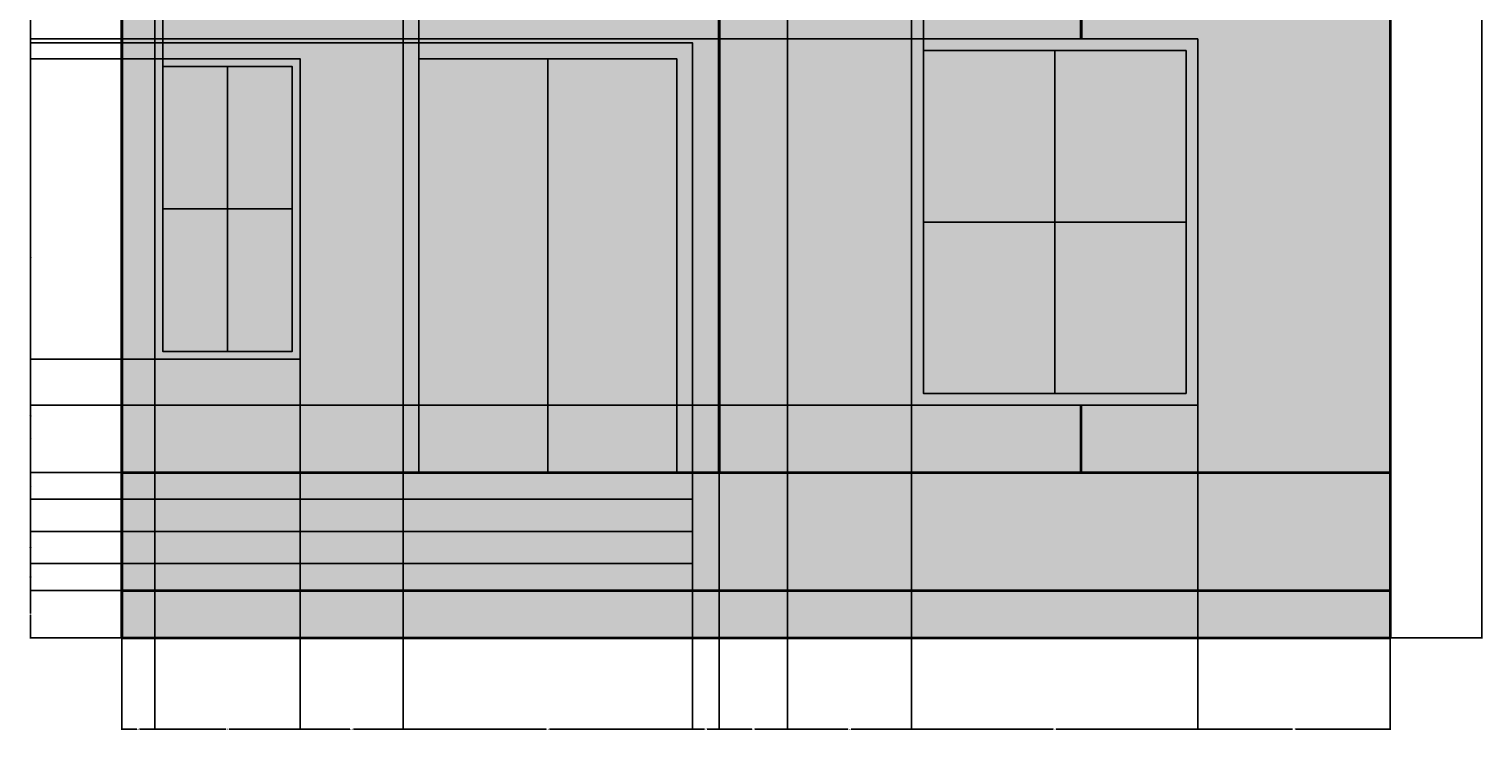
# Model space of a CAD drawing. Units: feet. Extents: x 2368 to 2738, y 1285 to 1782.
# Tile 1 of 6: x 2368 to 2738, y 1285 to 1464. Entities that reach past the tile are written whole.
import ezdxf

# ---------------------------------------------------------------- set-up
doc = ezdxf.new("R2010")
doc.units = ezdxf.units.FT
for name, color, linetype, lineweight in [('A-ANNO-DIMS', 2, 'Continuous', 18), ('A-DOOR', 3, 'Continuous', 25), ('A-ELEV', 7, 'Continuous', 35), ('A-ELEV-PATT', 252, 'Continuous', 13), ('A-FLOR-STRS', 2, 'Continuous', 25), ('A-GLAZ', 4, 'Continuous', 25)]:
    doc.layers.add(name, color=color, linetype=linetype, lineweight=lineweight)
doc.styles.get("Standard").update_dxf_attribs({"font": 'arial.ttf'})
doc.dimstyles.get("Standard").update_dxf_attribs({"dimtxt": 0.18, "dimasz": 0.18, "dimexe": 0.18, "dimexo": 0.0625, "dimgap": 0.09, "dimtad": 0, "dimtih": 1, "dimtoh": 1, "dimdec": 1, "dimzin": 0, "dimdsep": 46, "dimlunit": 3, "dimtxsty": 'Standard', "dimcen": 0.09, "dimadec": 0, "dimazin": 0, "dimtfac": 1, "dimtdec": 1, "dimtofl": 0, "dimtmove": 0, "dimatfit": 3, "dimfxl": 1, "dimtolj": 1, "dimtzin": 0, "dimarcsym": 0})

# ---------------------------------------------------------------- blocks, each defined once
blk = doc.blocks.new('*D2')
at = {"layer": 'A-ANNO-DIMS', "color": 0, "lineweight": -2, "transparency": 16777216}
for p, q in [((2714.23, 1758.68), (2737.59, 1758.68)), ((2737.41, 1758.5), (2737.41, 1533.95)), ((2737.41, 1309.04), (2737.41, 1533.58)), ((2714.23, 1308.86), (2737.59, 1308.86))]:
    blk.add_line(p, q, dxfattribs=at)
at = {"layer": 'A-ANNO-DIMS', "color": 0, "transparency": 16777216}
for points in [[(2737.38, 1758.5), (2737.44, 1758.5), (2737.41, 1758.68)], [(2737.38, 1309.04), (2737.44, 1309.04), (2737.41, 1308.86)]]:
    blk.add_solid(points, dxfattribs=at)
at = {"layer": 'Defpoints', "color": 0, "transparency": 16777216}
for p in [(2714.16, 1758.68), (2737.41, 1758.68), (2714.16, 1308.86)]:
    blk.add_point(p, dxfattribs=at)
at = {"layer": 'A-ANNO-DIMS', "color": 0, "transparency": 16777216, "insert": (2737.41, 1533.77), "char_height": 0.18, "attachment_point": 5}
blk.add_mtext('\\A1;449.8', dxfattribs=at)
blk = doc.blocks.new('*D3')
at = {"layer": 'A-ANNO-DIMS', "color": 0, "lineweight": -2, "transparency": 16777216}
for p, q in [((2391.48, 1320.86), (2368.11, 1320.86)), ((2368.29, 1320.68), (2368.29, 1315.04)), ((2368.29, 1309.04), (2368.29, 1314.67)), ((2391.48, 1308.86), (2368.11, 1308.86))]:
    blk.add_line(p, q, dxfattribs=at)
at = {"layer": 'A-ANNO-DIMS', "color": 0, "transparency": 16777216}
for points in [[(2368.26, 1320.68), (2368.32, 1320.68), (2368.29, 1320.86)], [(2368.26, 1309.04), (2368.32, 1309.04), (2368.29, 1308.86)]]:
    blk.add_solid(points, dxfattribs=at)
at = {"layer": 'Defpoints', "color": 0, "transparency": 16777216}
for p in [(2368.29, 1320.86), (2391.54, 1320.86), (2391.54, 1308.86)]:
    blk.add_point(p, dxfattribs=at)
at = {"layer": 'A-ANNO-DIMS', "color": 0, "transparency": 16777216, "insert": (2368.29, 1314.86), "char_height": 0.18, "attachment_point": 5}
blk.add_mtext('\\A1;12', dxfattribs=at)
blk = doc.blocks.new('*D4')
at = {"layer": 'A-ANNO-DIMS', "color": 0, "lineweight": -2, "transparency": 16777216}
for p, q in [((2391.48, 1350.86), (2368.11, 1350.86)), ((2368.29, 1350.68), (2368.29, 1336.04)), ((2368.29, 1321.04), (2368.29, 1335.67)), ((2391.48, 1320.86), (2368.11, 1320.86))]:
    blk.add_line(p, q, dxfattribs=at)
at = {"layer": 'A-ANNO-DIMS', "color": 0, "transparency": 16777216}
for points in [[(2368.26, 1350.68), (2368.32, 1350.68), (2368.29, 1350.86)], [(2368.26, 1321.04), (2368.32, 1321.04), (2368.29, 1320.86)]]:
    blk.add_solid(points, dxfattribs=at)
at = {"layer": 'Defpoints', "color": 0, "transparency": 16777216}
for p in [(2368.29, 1350.86), (2391.54, 1350.86), (2391.54, 1320.86)]:
    blk.add_point(p, dxfattribs=at)
at = {"layer": 'A-ANNO-DIMS', "color": 0, "transparency": 16777216, "insert": (2368.29, 1335.86), "char_height": 0.18, "attachment_point": 5}
blk.add_mtext('\\A1;30', dxfattribs=at)
blk = doc.blocks.new('*D5')
at = {"layer": 'A-ANNO-DIMS', "color": 0, "lineweight": -2, "transparency": 16777216}
for p, q in [((2399.84, 1379.67), (2368.11, 1379.67)), ((2368.29, 1379.49), (2368.29, 1365.44)), ((2368.29, 1351.04), (2368.29, 1365.08)), ((2391.48, 1350.86), (2368.11, 1350.86))]:
    blk.add_line(p, q, dxfattribs=at)
at = {"layer": 'A-ANNO-DIMS', "color": 0, "transparency": 16777216}
for points in [[(2368.26, 1379.49), (2368.32, 1379.49), (2368.29, 1379.67)], [(2368.26, 1351.04), (2368.32, 1351.04), (2368.29, 1350.86)]]:
    blk.add_solid(points, dxfattribs=at)
at = {"layer": 'Defpoints', "color": 0, "transparency": 16777216}
for p in [(2368.29, 1379.67), (2399.91, 1379.67), (2391.54, 1350.86)]:
    blk.add_point(p, dxfattribs=at)
at = {"layer": 'A-ANNO-DIMS', "color": 0, "transparency": 16777216, "insert": (2368.29, 1365.26), "char_height": 0.18, "attachment_point": 5}
blk.add_mtext('\\A1;28.814', dxfattribs=at)
blk = doc.blocks.new('*D6')
at = {"layer": 'A-ANNO-DIMS', "color": 0, "lineweight": -2, "transparency": 16777216}
for p, q in [((2391.48, 1482.86), (2368.11, 1482.86)), ((2368.29, 1482.68), (2368.29, 1469.65)), ((2368.29, 1456.26), (2368.29, 1469.29)), ((2399.84, 1456.08), (2368.11, 1456.08))]:
    blk.add_line(p, q, dxfattribs=at)
at = {"layer": 'A-ANNO-DIMS', "color": 0, "transparency": 16777216}
for points in [[(2368.26, 1482.68), (2368.32, 1482.68), (2368.29, 1482.86)], [(2368.26, 1456.26), (2368.32, 1456.26), (2368.29, 1456.08)]]:
    blk.add_solid(points, dxfattribs=at)
at = {"layer": 'Defpoints', "color": 0, "transparency": 16777216}
for p in [(2368.29, 1482.86), (2391.54, 1482.86), (2399.91, 1456.08)]:
    blk.add_point(p, dxfattribs=at)
at = {"layer": 'A-ANNO-DIMS', "color": 0, "transparency": 16777216, "insert": (2368.29, 1469.47), "char_height": 0.18, "attachment_point": 5}
blk.add_mtext('\\A1;26.77', dxfattribs=at)
blk = doc.blocks.new('*D14')
at = {"layer": 'A-ANNO-DIMS', "color": 0, "lineweight": -2, "transparency": 16777216}
for p, q in [((2399.91, 1379.61), (2399.91, 1285.43)), ((2391.54, 1350.79), (2391.54, 1285.43)), ((2391.72, 1285.61), (2395.33, 1285.61)), ((2399.73, 1285.61), (2396.12, 1285.61))]:
    blk.add_line(p, q, dxfattribs=at)
at = {"layer": 'A-ANNO-DIMS', "color": 0, "transparency": 16777216}
for points in [[(2391.72, 1285.64), (2391.72, 1285.58), (2391.54, 1285.61)], [(2399.73, 1285.64), (2399.73, 1285.58), (2399.91, 1285.61)]]:
    blk.add_solid(points, dxfattribs=at)
at = {"layer": 'Defpoints', "color": 0, "transparency": 16777216}
for p in [(2399.91, 1379.67), (2391.54, 1350.86), (2399.91, 1285.61)]:
    blk.add_point(p, dxfattribs=at)
at = {"layer": 'A-ANNO-DIMS', "color": 0, "transparency": 16777216, "insert": (2395.72, 1285.61), "char_height": 0.18, "attachment_point": 5}
blk.add_mtext('\\A1;8.365', dxfattribs=at)
blk = doc.blocks.new('*D15')
at = {"layer": 'A-ANNO-DIMS', "color": 0, "lineweight": -2, "transparency": 16777216}
for p, q in [((2399.91, 1379.61), (2399.91, 1285.43)), ((2436.85, 1379.61), (2436.85, 1285.43)), ((2400.09, 1285.61), (2417.98, 1285.61)), ((2436.67, 1285.61), (2418.77, 1285.61))]:
    blk.add_line(p, q, dxfattribs=at)
at = {"layer": 'A-ANNO-DIMS', "color": 0, "transparency": 16777216}
for points in [[(2400.09, 1285.64), (2400.09, 1285.58), (2399.91, 1285.61)], [(2436.67, 1285.64), (2436.67, 1285.58), (2436.85, 1285.61)]]:
    blk.add_solid(points, dxfattribs=at)
at = {"layer": 'Defpoints', "color": 0, "transparency": 16777216}
for p in [(2399.91, 1379.67), (2436.85, 1379.67), (2436.85, 1285.61)]:
    blk.add_point(p, dxfattribs=at)
at = {"layer": 'A-ANNO-DIMS', "color": 0, "transparency": 16777216, "insert": (2418.38, 1285.61), "char_height": 0.18, "attachment_point": 5}
blk.add_mtext('\\A1;36.94', dxfattribs=at)
blk = doc.blocks.new('*D16')
at = {"layer": 'A-ANNO-DIMS', "color": 0, "lineweight": -2, "transparency": 16777216}
for p, q in [((2436.85, 1379.61), (2436.85, 1285.43)), ((2463.03, 1350.79), (2463.03, 1285.43)), ((2437.03, 1285.61), (2449.48, 1285.61)), ((2462.85, 1285.61), (2450.41, 1285.61))]:
    blk.add_line(p, q, dxfattribs=at)
at = {"layer": 'A-ANNO-DIMS', "color": 0, "transparency": 16777216}
for points in [[(2437.03, 1285.64), (2437.03, 1285.58), (2436.85, 1285.61)], [(2462.85, 1285.64), (2462.85, 1285.58), (2463.03, 1285.61)]]:
    blk.add_solid(points, dxfattribs=at)
at = {"layer": 'Defpoints', "color": 0, "transparency": 16777216}
for p in [(2436.85, 1379.67), (2463.03, 1350.86), (2463.03, 1285.61)]:
    blk.add_point(p, dxfattribs=at)
at = {"layer": 'A-ANNO-DIMS', "color": 0, "transparency": 16777216, "insert": (2449.94, 1285.61), "char_height": 0.18, "attachment_point": 5}
blk.add_mtext('\\A1;26.184', dxfattribs=at)
blk = doc.blocks.new('*D17')
at = {"layer": 'A-ANNO-DIMS', "color": 0, "lineweight": -2, "transparency": 16777216}
for p, q in [((2463.03, 1350.79), (2463.03, 1285.43)), ((2536.68, 1350.79), (2536.68, 1285.43)), ((2463.21, 1285.61), (2499.46, 1285.61)), ((2536.5, 1285.61), (2500.25, 1285.61))]:
    blk.add_line(p, q, dxfattribs=at)
at = {"layer": 'A-ANNO-DIMS', "color": 0, "transparency": 16777216}
for points in [[(2463.21, 1285.64), (2463.21, 1285.58), (2463.03, 1285.61)], [(2536.5, 1285.64), (2536.5, 1285.58), (2536.68, 1285.61)]]:
    blk.add_solid(points, dxfattribs=at)
at = {"layer": 'Defpoints', "color": 0, "transparency": 16777216}
for p in [(2463.03, 1350.86), (2536.68, 1350.86), (2536.68, 1285.61)]:
    blk.add_point(p, dxfattribs=at)
at = {"layer": 'A-ANNO-DIMS', "color": 0, "transparency": 16777216, "insert": (2499.85, 1285.61), "char_height": 0.18, "attachment_point": 5}
blk.add_mtext('\\A1;73.64', dxfattribs=at)
blk = doc.blocks.new('*D18')
at = {"layer": 'A-ANNO-DIMS', "color": 0, "lineweight": -2, "transparency": 16777216}
for p, q in [((2536.68, 1350.79), (2536.68, 1285.43)), ((2543.45, 1350.79), (2543.45, 1285.43)), ((2536.86, 1285.61), (2539.74, 1285.61)), ((2543.27, 1285.61), (2540.39, 1285.61))]:
    blk.add_line(p, q, dxfattribs=at)
at = {"layer": 'A-ANNO-DIMS', "color": 0, "transparency": 16777216}
for points in [[(2536.86, 1285.64), (2536.86, 1285.58), (2536.68, 1285.61)], [(2543.27, 1285.64), (2543.27, 1285.58), (2543.45, 1285.61)]]:
    blk.add_solid(points, dxfattribs=at)
at = {"layer": 'Defpoints', "color": 0, "transparency": 16777216}
for p in [(2536.68, 1350.86), (2543.45, 1350.86), (2543.45, 1285.61)]:
    blk.add_point(p, dxfattribs=at)
at = {"layer": 'A-ANNO-DIMS', "color": 0, "transparency": 16777216, "insert": (2540.06, 1285.61), "char_height": 0.18, "attachment_point": 5}
blk.add_mtext('\\A1;6.77', dxfattribs=at)
blk = doc.blocks.new('*D19')
at = {"layer": 'A-ANNO-DIMS', "color": 0, "lineweight": -2, "transparency": 16777216}
for p, q in [((2560.8, 1466.04), (2560.8, 1285.43)), ((2543.45, 1350.79), (2543.45, 1285.43)), ((2543.63, 1285.61), (2551.74, 1285.61)), ((2560.62, 1285.61), (2552.51, 1285.61))]:
    blk.add_line(p, q, dxfattribs=at)
at = {"layer": 'A-ANNO-DIMS', "color": 0, "transparency": 16777216}
for points in [[(2543.63, 1285.64), (2543.63, 1285.58), (2543.45, 1285.61)], [(2560.62, 1285.64), (2560.62, 1285.58), (2560.8, 1285.61)]]:
    blk.add_solid(points, dxfattribs=at)
at = {"layer": 'Defpoints', "color": 0, "transparency": 16777216}
for p in [(2560.8, 1466.1), (2543.45, 1350.86), (2560.8, 1285.61)]:
    blk.add_point(p, dxfattribs=at)
at = {"layer": 'A-ANNO-DIMS', "color": 0, "transparency": 16777216, "insert": (2552.12, 1285.61), "char_height": 0.18, "attachment_point": 5}
blk.add_mtext('\\A1;17.35', dxfattribs=at)
blk = doc.blocks.new('*D20')
at = {"layer": 'A-ANNO-DIMS', "color": 0, "lineweight": -2, "transparency": 16777216}
for p, q in [((2560.8, 1466.04), (2560.8, 1285.43)), ((2592.41, 1367.92), (2592.41, 1285.43)), ((2560.98, 1285.61), (2576.21, 1285.61)), ((2592.23, 1285.61), (2577, 1285.61))]:
    blk.add_line(p, q, dxfattribs=at)
at = {"layer": 'A-ANNO-DIMS', "color": 0, "transparency": 16777216}
for points in [[(2560.98, 1285.64), (2560.98, 1285.58), (2560.8, 1285.61)], [(2592.23, 1285.64), (2592.23, 1285.58), (2592.41, 1285.61)]]:
    blk.add_solid(points, dxfattribs=at)
at = {"layer": 'Defpoints', "color": 0, "transparency": 16777216}
for p in [(2560.8, 1466.1), (2592.41, 1367.98), (2592.41, 1285.61)]:
    blk.add_point(p, dxfattribs=at)
at = {"layer": 'A-ANNO-DIMS', "color": 0, "transparency": 16777216, "insert": (2576.6, 1285.61), "char_height": 0.18, "attachment_point": 5}
blk.add_mtext('\\A1;31.62', dxfattribs=at)
blk = doc.blocks.new('*D21')
at = {"layer": 'A-ANNO-DIMS', "color": 0, "lineweight": -2, "transparency": 16777216}
for p, q in [((2592.41, 1367.92), (2592.41, 1285.43)), ((2665.2, 1367.92), (2665.2, 1285.43)), ((2592.59, 1285.61), (2628.41, 1285.61)), ((2665.02, 1285.61), (2629.2, 1285.61))]:
    blk.add_line(p, q, dxfattribs=at)
at = {"layer": 'A-ANNO-DIMS', "color": 0, "transparency": 16777216}
for points in [[(2592.59, 1285.64), (2592.59, 1285.58), (2592.41, 1285.61)], [(2665.02, 1285.64), (2665.02, 1285.58), (2665.2, 1285.61)]]:
    blk.add_solid(points, dxfattribs=at)
at = {"layer": 'Defpoints', "color": 0, "transparency": 16777216}
for p in [(2592.41, 1367.98), (2665.2, 1367.98), (2665.2, 1285.61)]:
    blk.add_point(p, dxfattribs=at)
at = {"layer": 'A-ANNO-DIMS', "color": 0, "transparency": 16777216, "insert": (2628.8, 1285.61), "char_height": 0.18, "attachment_point": 5}
blk.add_mtext('\\A1;72.78', dxfattribs=at)
blk = doc.blocks.new('*D22')
at = {"layer": 'A-ANNO-DIMS', "color": 0, "lineweight": -2, "transparency": 16777216}
for p, q in [((2665.2, 1367.92), (2665.2, 1285.43)), ((2714.16, 1350.79), (2714.16, 1285.43)), ((2665.38, 1285.61), (2689.28, 1285.61)), ((2713.98, 1285.61), (2690.08, 1285.61))]:
    blk.add_line(p, q, dxfattribs=at)
at = {"layer": 'A-ANNO-DIMS', "color": 0, "transparency": 16777216}
for points in [[(2665.38, 1285.64), (2665.38, 1285.58), (2665.2, 1285.61)], [(2713.98, 1285.64), (2713.98, 1285.58), (2714.16, 1285.61)]]:
    blk.add_solid(points, dxfattribs=at)
at = {"layer": 'Defpoints', "color": 0, "transparency": 16777216}
for p in [(2665.2, 1367.98), (2714.16, 1350.86), (2714.16, 1285.61)]:
    blk.add_point(p, dxfattribs=at)
at = {"layer": 'A-ANNO-DIMS', "color": 0, "transparency": 16777216, "insert": (2689.68, 1285.61), "char_height": 0.18, "attachment_point": 5}
blk.add_mtext('\\A1;48.97', dxfattribs=at)
blk = doc.blocks.new('*D23')
at = {"layer": 'A-ANNO-DIMS', "color": 0, "lineweight": -2, "transparency": 16777216}
for p, q in [((2399.84, 1456.08), (2368.11, 1456.08)), ((2368.29, 1455.9), (2368.29, 1418.06)), ((2368.29, 1379.85), (2368.29, 1417.69)), ((2399.84, 1379.67), (2368.11, 1379.67))]:
    blk.add_line(p, q, dxfattribs=at)
at = {"layer": 'A-ANNO-DIMS', "color": 0, "transparency": 16777216}
for points in [[(2368.26, 1455.9), (2368.32, 1455.9), (2368.29, 1456.08)], [(2368.26, 1379.85), (2368.32, 1379.85), (2368.29, 1379.67)]]:
    blk.add_solid(points, dxfattribs=at)
at = {"layer": 'Defpoints', "color": 0, "transparency": 16777216}
for p in [(2368.29, 1456.08), (2399.91, 1456.08), (2399.91, 1379.67)]:
    blk.add_point(p, dxfattribs=at)
at = {"layer": 'A-ANNO-DIMS', "color": 0, "transparency": 16777216, "insert": (2368.29, 1417.88), "char_height": 0.18, "attachment_point": 5}
blk.add_mtext('\\A1;76.42', dxfattribs=at)
blk = doc.blocks.new('*D24')
at = {"layer": 'A-ANNO-DIMS', "color": 0, "lineweight": -2, "transparency": 16777216}
for p, q in [((2399.91, 1456.15), (2399.91, 1782.11)), ((2400.09, 1781.93), (2400.76, 1781.93)), ((2401.73, 1781.93), (2401.06, 1781.93)), ((2401.91, 1454.15), (2401.91, 1782.11))]:
    blk.add_line(p, q, dxfattribs=at)
at = {"layer": 'A-ANNO-DIMS', "color": 0, "transparency": 16777216}
for points in [[(2400.09, 1781.96), (2400.09, 1781.9), (2399.91, 1781.93)], [(2401.73, 1781.96), (2401.73, 1781.9), (2401.91, 1781.93)]]:
    blk.add_solid(points, dxfattribs=at)
at = {"layer": 'Defpoints', "color": 0, "transparency": 16777216}
for p in [(2401.91, 1781.93), (2399.91, 1456.08), (2401.91, 1454.08)]:
    blk.add_point(p, dxfattribs=at)
at = {"layer": 'A-ANNO-DIMS', "color": 0, "transparency": 16777216, "insert": (2400.91, 1781.93), "char_height": 0.18, "attachment_point": 5}
blk.add_mtext('\\A1;2', dxfattribs=at)
blk = doc.blocks.new('*D25')
at = {"layer": 'A-ANNO-DIMS', "color": 0, "lineweight": -2, "transparency": 16777216}
for p, q in [((2462.97, 1327.76), (2368.11, 1327.76)), ((2368.29, 1327.58), (2368.29, 1324.49)), ((2368.29, 1321.04), (2368.29, 1324.12)), ((2462.97, 1320.86), (2368.11, 1320.86))]:
    blk.add_line(p, q, dxfattribs=at)
at = {"layer": 'A-ANNO-DIMS', "color": 0, "transparency": 16777216}
for points in [[(2368.26, 1327.58), (2368.32, 1327.58), (2368.29, 1327.76)], [(2368.26, 1321.04), (2368.32, 1321.04), (2368.29, 1320.86)]]:
    blk.add_solid(points, dxfattribs=at)
at = {"layer": 'Defpoints', "color": 0, "transparency": 16777216}
for p in [(2368.29, 1327.76), (2463.03, 1327.76), (2463.03, 1320.86)]:
    blk.add_point(p, dxfattribs=at)
at = {"layer": 'A-ANNO-DIMS', "color": 0, "transparency": 16777216, "insert": (2368.29, 1324.31), "char_height": 0.18, "attachment_point": 5}
blk.add_mtext('\\A1;6.901', dxfattribs=at)
blk = doc.blocks.new('*D26')
at = {"layer": 'A-ANNO-DIMS', "color": 0, "lineweight": -2, "transparency": 16777216}
for p, q in [((2462.97, 1335.86), (2368.11, 1335.86)), ((2368.29, 1335.68), (2368.29, 1331.99)), ((2368.29, 1327.94), (2368.29, 1331.62)), ((2462.97, 1327.76), (2368.11, 1327.76))]:
    blk.add_line(p, q, dxfattribs=at)
at = {"layer": 'A-ANNO-DIMS', "color": 0, "transparency": 16777216}
for points in [[(2368.26, 1335.68), (2368.32, 1335.68), (2368.29, 1335.86)], [(2368.26, 1327.94), (2368.32, 1327.94), (2368.29, 1327.76)]]:
    blk.add_solid(points, dxfattribs=at)
at = {"layer": 'Defpoints', "color": 0, "transparency": 16777216}
for p in [(2368.29, 1335.86), (2463.03, 1335.86), (2463.03, 1327.76)]:
    blk.add_point(p, dxfattribs=at)
at = {"layer": 'A-ANNO-DIMS', "color": 0, "transparency": 16777216, "insert": (2368.29, 1331.81), "char_height": 0.18, "attachment_point": 5}
blk.add_mtext('\\A1;8.099', dxfattribs=at)
blk = doc.blocks.new('*D27')
at = {"layer": 'A-ANNO-DIMS', "color": 0, "lineweight": -2, "transparency": 16777216}
for p, q in [((2462.97, 1344.11), (2368.11, 1344.11)), ((2368.29, 1343.93), (2368.29, 1340.17)), ((2368.29, 1336.04), (2368.29, 1339.8)), ((2462.97, 1335.86), (2368.11, 1335.86))]:
    blk.add_line(p, q, dxfattribs=at)
at = {"layer": 'A-ANNO-DIMS', "color": 0, "transparency": 16777216}
for points in [[(2368.26, 1343.93), (2368.32, 1343.93), (2368.29, 1344.11)], [(2368.26, 1336.04), (2368.32, 1336.04), (2368.29, 1335.86)]]:
    blk.add_solid(points, dxfattribs=at)
at = {"layer": 'Defpoints', "color": 0, "transparency": 16777216}
for p in [(2368.29, 1344.11), (2463.03, 1344.11), (2463.03, 1335.86)]:
    blk.add_point(p, dxfattribs=at)
at = {"layer": 'A-ANNO-DIMS', "color": 0, "transparency": 16777216, "insert": (2368.29, 1339.98), "char_height": 0.18, "attachment_point": 5}
blk.add_mtext('\\A1;8.258', dxfattribs=at)
blk = doc.blocks.new('*D28')
at = {"layer": 'A-ANNO-DIMS', "color": 0, "lineweight": -2, "transparency": 16777216}
for p, q in [((2462.97, 1350.86), (2368.11, 1350.86)), ((2368.29, 1350.68), (2368.29, 1347.67)), ((2368.29, 1344.29), (2368.29, 1347.3)), ((2462.97, 1344.11), (2368.11, 1344.11))]:
    blk.add_line(p, q, dxfattribs=at)
at = {"layer": 'A-ANNO-DIMS', "color": 0, "transparency": 16777216}
for points in [[(2368.26, 1350.68), (2368.32, 1350.68), (2368.29, 1350.86)], [(2368.26, 1344.29), (2368.32, 1344.29), (2368.29, 1344.11)]]:
    blk.add_solid(points, dxfattribs=at)
at = {"layer": 'Defpoints', "color": 0, "transparency": 16777216}
for p in [(2368.29, 1350.86), (2463.03, 1350.86), (2463.03, 1344.11)]:
    blk.add_point(p, dxfattribs=at)
at = {"layer": 'A-ANNO-DIMS', "color": 0, "transparency": 16777216, "insert": (2368.29, 1347.48), "char_height": 0.18, "attachment_point": 5}
blk.add_mtext('\\A1;6.742', dxfattribs=at)
blk = doc.blocks.new('*D29')
at = {"layer": 'A-ANNO-DIMS', "color": 0, "lineweight": -2, "transparency": 16777216}
for p, q in [((2462.97, 1460.1), (2368.11, 1460.1)), ((2368.29, 1459.92), (2368.29, 1405.66)), ((2368.29, 1351.04), (2368.29, 1405.29)), ((2462.97, 1350.86), (2368.11, 1350.86))]:
    blk.add_line(p, q, dxfattribs=at)
at = {"layer": 'A-ANNO-DIMS', "color": 0, "transparency": 16777216}
for points in [[(2368.26, 1459.92), (2368.32, 1459.92), (2368.29, 1460.1)], [(2368.26, 1351.04), (2368.32, 1351.04), (2368.29, 1350.86)]]:
    blk.add_solid(points, dxfattribs=at)
at = {"layer": 'Defpoints', "color": 0, "transparency": 16777216}
for p in [(2368.29, 1460.1), (2463.03, 1460.1), (2463.03, 1350.86)]:
    blk.add_point(p, dxfattribs=at)
at = {"layer": 'A-ANNO-DIMS', "color": 0, "transparency": 16777216, "insert": (2368.29, 1405.48), "char_height": 0.18, "attachment_point": 5}
blk.add_mtext('\\A1;109.24', dxfattribs=at)
blk = doc.blocks.new('*D30')
at = {"layer": 'A-ANNO-DIMS', "color": 0, "lineweight": -2, "transparency": 16777216}
for p, q in [((2463.03, 1460.16), (2463.03, 1782.11)), ((2463.21, 1781.93), (2464.88, 1781.93)), ((2466.85, 1781.93), (2465.18, 1781.93)), ((2467.03, 1456.16), (2467.03, 1782.11))]:
    blk.add_line(p, q, dxfattribs=at)
at = {"layer": 'A-ANNO-DIMS', "color": 0, "transparency": 16777216}
for points in [[(2463.21, 1781.96), (2463.21, 1781.9), (2463.03, 1781.93)], [(2466.85, 1781.96), (2466.85, 1781.9), (2467.03, 1781.93)]]:
    blk.add_solid(points, dxfattribs=at)
at = {"layer": 'Defpoints', "color": 0, "transparency": 16777216}
for p in [(2467.03, 1781.93), (2463.03, 1460.1), (2467.03, 1456.1)]:
    blk.add_point(p, dxfattribs=at)
at = {"layer": 'A-ANNO-DIMS', "color": 0, "transparency": 16777216, "insert": (2465.03, 1781.93), "char_height": 0.18, "attachment_point": 5}
blk.add_mtext('\\A1;4', dxfattribs=at)
blk = doc.blocks.new('*D31')
at = {"layer": 'A-ANNO-DIMS', "color": 0, "lineweight": -2, "transparency": 16777216}
for p, q in [((2592.35, 1367.98), (2368.11, 1367.98)), ((2368.29, 1367.8), (2368.29, 1359.6)), ((2368.29, 1351.04), (2368.29, 1359.24)), ((2635.43, 1350.86), (2368.11, 1350.86))]:
    blk.add_line(p, q, dxfattribs=at)
at = {"layer": 'A-ANNO-DIMS', "color": 0, "transparency": 16777216}
for points in [[(2368.26, 1367.8), (2368.32, 1367.8), (2368.29, 1367.98)], [(2368.26, 1351.04), (2368.32, 1351.04), (2368.29, 1350.86)]]:
    blk.add_solid(points, dxfattribs=at)
at = {"layer": 'Defpoints', "color": 0, "transparency": 16777216}
for p in [(2368.29, 1367.98), (2592.41, 1367.98), (2635.49, 1350.86)]:
    blk.add_point(p, dxfattribs=at)
at = {"layer": 'A-ANNO-DIMS', "color": 0, "transparency": 16777216, "insert": (2368.29, 1359.42), "char_height": 0.18, "attachment_point": 5}
blk.add_mtext('\\A1;17.13', dxfattribs=at)
blk = doc.blocks.new('*D32')
at = {"layer": 'A-ANNO-DIMS', "color": 0, "lineweight": -2, "transparency": 16777216}
for p, q in [((2592.35, 1461.14), (2368.11, 1461.14)), ((2368.29, 1460.96), (2368.29, 1414.74)), ((2368.29, 1368.16), (2368.29, 1414.38)), ((2592.35, 1367.98), (2368.11, 1367.98))]:
    blk.add_line(p, q, dxfattribs=at)
at = {"layer": 'A-ANNO-DIMS', "color": 0, "transparency": 16777216}
for points in [[(2368.26, 1460.96), (2368.32, 1460.96), (2368.29, 1461.14)], [(2368.26, 1368.16), (2368.32, 1368.16), (2368.29, 1367.98)]]:
    blk.add_solid(points, dxfattribs=at)
at = {"layer": 'Defpoints', "color": 0, "transparency": 16777216}
for p in [(2368.29, 1461.14), (2592.41, 1461.14), (2592.41, 1367.98)]:
    blk.add_point(p, dxfattribs=at)
at = {"layer": 'A-ANNO-DIMS', "color": 0, "transparency": 16777216, "insert": (2368.29, 1414.56), "char_height": 0.18, "attachment_point": 5}
blk.add_mtext('\\A1;93.16', dxfattribs=at)
blk = doc.blocks.new('*D33')
at = {"layer": 'A-ANNO-DIMS', "color": 0, "lineweight": -2, "transparency": 16777216}
for p, q in [((2592.41, 1461.2), (2592.41, 1782.11)), ((2592.59, 1781.93), (2593.76, 1781.93)), ((2595.23, 1781.93), (2594.06, 1781.93)), ((2595.41, 1458.2), (2595.41, 1782.11))]:
    blk.add_line(p, q, dxfattribs=at)
at = {"layer": 'A-ANNO-DIMS', "color": 0, "transparency": 16777216}
for points in [[(2592.59, 1781.96), (2592.59, 1781.9), (2592.41, 1781.93)], [(2595.23, 1781.96), (2595.23, 1781.9), (2595.41, 1781.93)]]:
    blk.add_solid(points, dxfattribs=at)
at = {"layer": 'Defpoints', "color": 0, "transparency": 16777216}
for p in [(2595.41, 1781.93), (2592.41, 1461.14), (2595.41, 1458.14)]:
    blk.add_point(p, dxfattribs=at)
at = {"layer": 'A-ANNO-DIMS', "color": 0, "transparency": 16777216, "insert": (2593.91, 1781.93), "char_height": 0.18, "attachment_point": 5}
blk.add_mtext('\\A1;3', dxfattribs=at)

msp = doc.modelspace()

# ---------------------------------------------------------------- hatches: boundary and pattern name
at = {"layer": 'A-ELEV-PATT'}
h = msp.add_hatch(color=256, dxfattribs=at)
h.set_gradient(color1=(192, 192, 192), color2=(192, 192, 192), tint=1)
h.paths.add_polyline_path([(2714.1625, 1758.6751), (2519.621, 1758.6751), (2519.621, 1716.8552), (2714.1625, 1716.8552)])
h.paths.add_polyline_path([(2701.6591, 1693.9847), (2714.1625, 1693.9847), (2714.1625, 1710.8552), (2519.621, 1710.8552), (2519.621, 1662.8552), (2592.4132, 1662.8552), (2592.4132, 1689.493), (2665.1962, 1689.493), (2665.1962, 1662.8552), (2701.6591, 1662.8552)])
h.paths.add_polyline_path([(2701.6591, 1609.9058), (2597.776, 1609.9058), (2597.776, 1600.4784), (2665.1962, 1600.4784), (2665.1962, 1596.3371), (2665.1962, 1522.6314), (2701.6591, 1522.6314)])
h.paths.add_polyline_path([(2463.0324, 1598.097), (2536.677, 1598.097), (2536.677, 1519.7115), (2560.74, 1519.7115), (2560.5754, 1609.9058), (2542.3749, 1609.9058), (2441.2488, 1609.9058), (2441.2488, 1519.7115), (2463.0324, 1519.7115)])
h.paths.add_polyline_path([(2506.1956, 1662.8552), (2391.5414, 1662.8552), (2391.5414, 1644.4206), (2438.815, 1644.4206, -0.34592239), (2445.9507, 1638.8128), (2506.1956, 1638.8128)])
h.paths.add_polyline_path([(2410.9473, 1609.9058, -0.04175491), (2411.9608, 1614.8552), (2391.5414, 1614.8552), (2391.5414, 1488.8552), (2410.9473, 1488.8552)])
h.paths.add_polyline_path([(2426.5897, 1605.0962, 1), (2422.7862, 1605.0962), (2422.7862, 1509.5049, 1), (2426.5897, 1509.5049)])
h.paths.add_polyline_path([(2463.0324, 1460.097), (2536.677, 1460.097), (2536.677, 1350.8552), (2543.4468, 1350.8552), (2543.4468, 1482.8552), (2391.5414, 1482.8552), (2391.5414, 1350.8552), (2463.0324, 1350.8552)])
h.paths.add_polyline_path([(2436.8485, 1456.084), (2436.8485, 1379.669), (2399.9065, 1379.669), (2399.9065, 1456.084)], flags=16)
h.paths.add_polyline_path([(2434.8485, 1454.084), (2434.8485, 1381.669), (2401.9065, 1381.669), (2401.9065, 1454.084)], flags=0)
h.paths.add_polyline_path([(2714.1625, 1350.8552), (2391.5414, 1350.8552), (2391.5414, 1320.8552), (2714.1625, 1320.8552)])
h.paths.add_polyline_path([(2714.1625, 1320.8552), (2391.5414, 1320.8552), (2391.5414, 1308.8552), (2714.1625, 1308.8552)])
h = msp.add_hatch(color=256, dxfattribs=at)
h.set_gradient(color1=(0, 255, 255), color2=(0, 255, 255), tint=1)
h.paths.add_polyline_path([(2418.2281, 1454.084), (2401.9065, 1454.084), (2401.9065, 1381.669), (2418.2281, 1381.669)])
h.paths.add_polyline_path([(2434.8485, 1454.084), (2418.5148, 1454.084), (2418.5148, 1381.669), (2434.8485, 1381.669)])
h.paths.add_polyline_path([(2662.1962, 1458.1396), (2595.4132, 1458.1396), (2595.4132, 1414.5617), (2662.1962, 1414.5617)])
h.paths.add_polyline_path([(2662.1962, 1414.5617), (2628.8047, 1414.5617), (2628.8047, 1370.9838), (2662.1962, 1370.9838)])
h.paths.add_polyline_path([(2628.8047, 1414.5617), (2595.4132, 1414.5617), (2595.4132, 1370.9838), (2628.8047, 1370.9838)])
h.paths.add_polyline_path([(2662.1962, 1597.4784), (2628.8047, 1597.4784), (2628.8047, 1553.9004), (2662.1962, 1553.9004)])
h.paths.add_polyline_path([(2628.8047, 1597.4784), (2597.776, 1597.4784), (2597.776, 1553.9004), (2628.8047, 1553.9004)])
h.paths.add_polyline_path([(2628.8047, 1553.9004), (2597.776, 1553.9004), (2597.776, 1522.6314), (2628.8047, 1522.6314)])
h.paths.add_polyline_path([(2662.1962, 1553.9004), (2628.8047, 1553.9004), (2628.8047, 1522.6314), (2662.1962, 1522.6314)])
h.paths.add_polyline_path([(2662.1962, 1686.493), (2628.8047, 1686.493), (2628.8047, 1662.8552), (2662.1962, 1662.8552)])
h.paths.add_polyline_path([(2628.8047, 1686.493), (2595.4132, 1686.493), (2595.4132, 1662.8552), (2628.8047, 1662.8552)])
h = msp.add_hatch(color=256, dxfattribs=at)
h.set_gradient(color1=(255, 255, 255), tint=1)
h.paths.add_polyline_path([(2595.4132, 1686.493), (2662.1962, 1686.493), (2662.1962, 1662.8552), (2665.1962, 1662.8552), (2665.1962, 1689.493), (2592.4132, 1689.493), (2592.4132, 1662.8552), (2595.4132, 1662.8552)])
h.paths.add_polyline_path([(2665.1962, 1600.4784), (2597.776, 1600.4784), (2597.776, 1597.4784), (2662.1962, 1597.4784), (2662.1962, 1510.3225), (2597.776, 1510.3225), (2597.776, 1507.3225), (2665.1962, 1507.3225)])
h.paths.add_polyline_path([(2665.1962, 1461.1396), (2592.4132, 1461.1396), (2592.4132, 1367.9838), (2665.1962, 1367.9838)])
h.paths.add_polyline_path([(2662.1962, 1458.1396), (2662.1962, 1370.9838), (2595.4132, 1370.9838), (2595.4132, 1458.1396)], flags=16)
h.paths.add_polyline_path([(2593.776, 1609.9058), (2584.2358, 1609.9058), (2584.2358, 1488.8552), (2593.776, 1488.8552)])
h.paths.add_polyline_path([(2597.776, 1609.9058), (2595.4517, 1609.9058), (2595.4517, 1488.8552), (2597.776, 1488.8552)])
h.paths.add_polyline_path([(2569.8357, 1609.9058), (2560.5754, 1609.9058), (2560.74, 1519.7115), (2560.7407, 1519.7115), (2560.7407, 1519.3328), (2560.7963, 1488.8552), (2569.8357, 1488.8552)])
h.paths.add_polyline_path([(2572.6807, 1609.9058), (2571.6967, 1609.9058), (2571.6967, 1488.8552), (2572.6807, 1488.8552)])
h.paths.add_polyline_path([(2575.8428, 1609.9058), (2574.5416, 1609.9058), (2574.5416, 1488.8552), (2575.8428, 1488.8552)])
h.paths.add_polyline_path([(2579.0308, 1609.9058), (2577.7037, 1609.9058), (2577.7037, 1488.8552), (2579.0308, 1488.8552)])
h.paths.add_polyline_path([(2582.3749, 1609.9058), (2580.8918, 1609.9058), (2580.8918, 1488.8552), (2582.3749, 1488.8552)])
h = msp.add_hatch(color=256, dxfattribs=at)
h.set_gradient(color1=(242, 242, 242), color2=(242, 242, 242), tint=1)
h.paths.add_polyline_path([(2542.3749, 1636.6235), (2440.8236, 1636.6235, 0.37790365), (2410.9473, 1609.9058), (2410.9473, 1488.8552), (2441.2488, 1488.8552), (2441.2488, 1609.9058), (2542.3749, 1609.9058)])
h.paths.add_polyline_path([(2426.5897, 1605.0962), (2426.5897, 1509.5049, -1), (2422.7862, 1509.5049), (2422.7862, 1605.0962, -1)], flags=16)
h.paths.add_polyline_path([(2441.2488, 1636.6235), (2446.1448, 1636.6235, 0.43242195), (2438.815, 1644.4206), (2391.5414, 1644.4206), (2391.5414, 1620.8552), (2391.5414, 1614.8552), (2411.9608, 1614.8552, -0.33482359)])
h.paths.add_polyline_path([(2592.4132, 1461.1396), (2635.4878, 1461.1396), (2635.4878, 1466.101), (2560.7963, 1466.101), (2560.7963, 1482.8552), (2543.4468, 1482.8552), (2543.4468, 1350.8552), (2635.4878, 1350.8552), (2635.4878, 1367.9838), (2592.4132, 1367.9838)])
h = msp.add_hatch(color=256, dxfattribs=at)
h.set_gradient(color2=(0, 0, 0), tint=1)
h.paths.add_polyline_path([(2467.0324, 1594.097), (2532.677, 1594.097), (2532.677, 1519.7115), (2536.677, 1519.7115), (2536.677, 1598.097), (2463.0324, 1598.097), (2463.0324, 1519.7115), (2467.0324, 1519.7115)])
h.paths.add_polyline_path([(2536.677, 1460.097), (2463.0324, 1460.097), (2463.0324, 1350.8552), (2467.0324, 1350.8552), (2467.0324, 1456.097), (2532.677, 1456.097), (2532.677, 1350.8552), (2536.677, 1350.8552)])
h.paths.add_polyline_path([(2436.8485, 1456.084), (2399.9065, 1456.084), (2399.9065, 1379.669), (2436.8485, 1379.669)])
h.paths.add_polyline_path([(2401.9065, 1454.084), (2434.8485, 1454.084), (2434.8485, 1381.669), (2401.9065, 1381.669)], flags=16)
h = msp.add_hatch(color=256, dxfattribs=at)
h.set_gradient(color1=(89, 52, 3), color2=(89, 52, 3), tint=1)
h.paths.add_polyline_path([(2532.677, 1456.097), (2499.8547, 1456.097), (2499.8547, 1350.8552), (2532.677, 1350.8552)])
h.paths.add_polyline_path([(2499.8547, 1456.097), (2467.0324, 1456.097), (2467.0324, 1350.8552), (2499.8547, 1350.8552)])
h.paths.add_polyline_path([(2499.8547, 1594.097), (2467.0324, 1594.097), (2467.0324, 1519.7115), (2499.8547, 1519.7115)])
h.paths.add_polyline_path([(2532.677, 1594.097), (2499.8547, 1594.097), (2499.8547, 1519.7115), (2532.677, 1519.7115)])
h = msp.add_hatch(color=256, dxfattribs=at)
h.set_gradient(color1=(144, 103, 100), color2=(144, 103, 100), tint=1)
h.paths.add_polyline_path([(2714.1625, 1466.101), (2701.6591, 1466.101), (2635.4878, 1466.101), (2635.4878, 1461.1396), (2665.1962, 1461.1396), (2665.1962, 1367.9838), (2635.4878, 1367.9838), (2635.4878, 1350.8552), (2714.1625, 1350.8552)])

# ---------------------------------------------------------------- linework, layer by layer
at = {"layer": 'A-DOOR'}
for p, q in [((2499.8547, 1456.097), (2499.8547, 1350.8552)), ((2499.8547, 1350.8552), (2499.8547, 1456.097)), ((2499.8547, 1456.097), (2499.8547, 1350.8552))]:
    msp.add_line(p, q, dxfattribs=at)
for points in [[(2536.677, 1350.8552), (2536.677, 1460.097), (2463.0324, 1460.097), (2463.0324, 1350.8552)], [(2532.677, 1350.8552), (2532.677, 1456.097), (2467.0324, 1456.097), (2467.0324, 1350.8552)]]:
    msp.add_lwpolyline(points, dxfattribs=at)
msp.add_lwpolyline([(2499.8547, 1456.097), (2499.8547, 1456.097), (2499.8547, 1350.8552), (2499.8547, 1350.8552)], close=True, dxfattribs=at)
at = {"layer": 'A-ELEV'}
for p, q in [((2391.5414, 1644.4206), (2391.5414, 1308.8552)), ((2391.5414, 1350.8552), (2391.5414, 1482.8552)), ((2543.4468, 1350.8552), (2543.4468, 1482.8552)), ((2543.4468, 1482.8552), (2543.4468, 1350.8552)), ((2635.4878, 1461.1396), (2635.4878, 1466.101)), ((2635.4878, 1466.101), (2635.4878, 1461.1396)), ((2635.4878, 1350.8552), (2635.4878, 1367.9838)), ((2635.4878, 1350.8552), (2635.4878, 1367.9838)), ((2391.5414, 1320.8552), (2391.5414, 1350.8552)), ((2391.5414, 1350.8552), (2714.1625, 1350.8552)), ((2391.5414, 1350.8552), (2714.1625, 1350.8552)), ((2391.5414, 1308.8552), (2391.5414, 1320.8552)), ((2391.5414, 1320.8552), (2714.1625, 1320.8552)), ((2391.5414, 1320.8552), (2714.1625, 1320.8552)), ((2391.5414, 1308.8552), (2714.1625, 1308.8552))]:
    msp.add_line(p, q, dxfattribs=at)
msp.add_lwpolyline([(2714.1625, 1716.8552), (2714.1625, 1308.8552)], dxfattribs=at)
at = {"layer": 'A-FLOR-STRS'}
for p, q in [((2463.0324, 1350.8552), (2463.0324, 1320.8552)), ((2536.677, 1350.8552), (2536.677, 1320.8552)), ((2463.0324, 1344.1131), (2536.677, 1344.1131)), ((2463.0324, 1335.8552), (2536.677, 1335.8552)), ((2463.0324, 1327.7563), (2536.677, 1327.7563))]:
    msp.add_line(p, q, dxfattribs=at)
at = {"layer": 'A-GLAZ'}
for p, q in [((2635.4878, 1461.1396), (2592.4132, 1461.1396)), ((2592.4132, 1461.1396), (2592.4132, 1367.9838)), ((2665.1962, 1461.1396), (2635.4878, 1461.1396)), ((2665.1962, 1367.9838), (2665.1962, 1461.1396)), ((2628.8047, 1370.9838), (2628.8047, 1458.1396)), ((2418.3775, 1454.084), (2418.3775, 1381.669)), ((2418.3775, 1454.084), (2418.3775, 1381.669)), ((2401.9065, 1417.8765), (2434.8485, 1417.8765)), ((2595.4132, 1414.5617), (2662.1962, 1414.5617)), ((2592.4132, 1367.9838), (2665.1962, 1367.9838))]:
    msp.add_line(p, q, dxfattribs=at)
for points in [[(2592.4132, 1461.1396), (2665.1962, 1461.1396), (2665.1962, 1367.9838), (2592.4132, 1367.9838)], [(2595.4132, 1458.1396), (2662.1962, 1458.1396), (2662.1962, 1370.9838), (2595.4132, 1370.9838)], [(2595.4132, 1458.1396), (2662.1962, 1458.1396), (2662.1962, 1370.9838), (2595.4132, 1370.9838)], [(2628.8047, 1370.9838), (2628.8047, 1370.9838), (2628.8047, 1458.1396), (2628.8047, 1458.1396)], [(2399.9065, 1456.084), (2436.8485, 1456.084), (2436.8485, 1379.669), (2399.9065, 1379.669)], [(2401.9065, 1454.084), (2434.8485, 1454.084), (2434.8485, 1381.669), (2401.9065, 1381.669)], [(2595.4132, 1414.5617), (2662.1962, 1414.5617), (2662.1962, 1414.5617), (2595.4132, 1414.5617)]]:
    msp.add_lwpolyline(points, close=True, dxfattribs=at)

# ---------------------------------------------------------------- dimensions: what is measured, and where the dimension line sits
at = {"layer": 'A-ANNO-DIMS'}
for base, p1, p2, override, picture, middle in [((2401.9065, 1781.9251), (2399.9065, 1456.084), (2401.9065, 1454.084), {"dimdec": 0, "dimlfac": 1, "dimrnd": 0, "dimzin": 0, "dimdsep": 46, "dimlunit": 2}, '*D24', (2400.9065, 1781.9251)), ((2467.0324, 1781.9251), (2463.0324, 1460.097), (2467.0324, 1456.097), {"dimdec": 0, "dimlfac": 1, "dimrnd": 0, "dimzin": 0, "dimdsep": 46, "dimlunit": 2}, '*D30', (2465.0324, 1781.9251)), ((2595.4132, 1781.9251), (2592.4132, 1461.1396), (2595.4132, 1458.1396), {"dimdec": 0, "dimlfac": 1, "dimrnd": 0, "dimzin": 0, "dimdsep": 46, "dimlunit": 2}, '*D33', (2593.9132, 1781.9251)), ((2560.7963, 1285.6052), (2543.4468, 1350.8552), (2560.7963, 1466.101), {"dimdec": 2, "dimlfac": 1, "dimrnd": 0, "dimzin": 0, "dimdsep": 46, "dimlunit": 2}, '*D19', (2552.1216, 1285.6052)), ((2592.4132, 1285.6052), (2560.7963, 1466.101), (2592.4132, 1367.9838), {"dimdec": 2, "dimlfac": 1, "dimrnd": 0, "dimzin": 0, "dimdsep": 46, "dimlunit": 2}, '*D20', (2576.6047, 1285.6052)), ((2399.9065, 1285.6052), (2391.5414, 1350.8552), (2399.9065, 1379.669), {"dimdec": 3, "dimlfac": 1, "dimrnd": 0, "dimzin": 0, "dimdsep": 46, "dimlunit": 2}, '*D14', (2395.7239, 1285.6052)), ((2436.8485, 1285.6052), (2399.9065, 1379.669), (2436.8485, 1379.669), {"dimdec": 2, "dimlfac": 1, "dimrnd": 0, "dimzin": 0, "dimdsep": 46, "dimlunit": 2}, '*D15', (2418.3775, 1285.6052)), ((2463.0324, 1285.6052), (2436.8485, 1379.669), (2463.0324, 1350.8552), {"dimdec": 3, "dimlfac": 1, "dimrnd": 0, "dimzin": 0, "dimdsep": 46, "dimlunit": 2}, '*D16', (2449.9405, 1285.6052)), ((2665.1962, 1285.6052), (2592.4132, 1367.9838), (2665.1962, 1367.9838), {"dimdec": 2, "dimlfac": 1, "dimrnd": 0, "dimzin": 0, "dimdsep": 46, "dimlunit": 2}, '*D21', (2628.8047, 1285.6052)), ((2714.1625, 1285.6052), (2665.1962, 1367.9838), (2714.1625, 1350.8552), {"dimdec": 2, "dimlfac": 1, "dimrnd": 0, "dimzin": 0, "dimdsep": 46, "dimlunit": 2}, '*D22', (2689.6793, 1285.6052)), ((2536.677, 1285.6052), (2463.0324, 1350.8552), (2536.677, 1350.8552), {"dimdec": 2, "dimlfac": 1, "dimrnd": 0, "dimzin": 0, "dimdsep": 46, "dimlunit": 2}, '*D17', (2499.8547, 1285.6052)), ((2543.4468, 1285.6052), (2536.677, 1350.8552), (2543.4468, 1350.8552), {"dimdec": 2, "dimlfac": 1, "dimrnd": 0, "dimzin": 0, "dimdsep": 46, "dimlunit": 2}, '*D18', (2540.0619, 1285.6052))]:
    dim = msp.add_linear_dim(base=base, p1=p1, p2=p2, dimstyle='Standard', override=override, dxfattribs=at)
    dim.commit()
    dim.dimension.update_dxf_attribs({"geometry": picture, "text_midpoint": middle})
for base, p1, p2, override, picture, middle in [((2737.4125, 1758.6751), (2714.1625, 1308.8552), (2714.1625, 1758.6751), {"dimdec": 1, "dimlfac": 1, "dimrnd": 0, "dimzin": 0, "dimdsep": 46, "dimlunit": 2}, '*D2', (2737.4125, 1533.7652)), ((2368.2914, 1482.8552), (2399.9065, 1456.084), (2391.5414, 1482.8552), {"dimdec": 2, "dimlfac": 1, "dimrnd": 0, "dimzin": 0, "dimdsep": 46, "dimlunit": 2}, '*D6', (2368.2914, 1469.4696)), ((2368.2914, 1461.1396), (2592.4132, 1367.9838), (2592.4132, 1461.1396), {"dimdec": 2, "dimlfac": 1, "dimrnd": 0, "dimzin": 0, "dimdsep": 46, "dimlunit": 2}, '*D32', (2368.2914, 1414.5617)), ((2368.2914, 1460.097), (2463.0324, 1350.8552), (2463.0324, 1460.097), {"dimdec": 2, "dimlfac": 1, "dimrnd": 0, "dimzin": 0, "dimdsep": 46, "dimlunit": 2}, '*D29', (2368.2914, 1405.4761)), ((2368.29138, 1456.08404), (2399.90647, 1379.66895), (2399.90647, 1456.08404), {"dimdec": 2, "dimlfac": 1, "dimrnd": 0, "dimzin": 0, "dimdsep": 46, "dimlunit": 2}, '*D23', (2368.29138, 1417.87649)), ((2368.2914, 1379.669), (2391.5414, 1350.8552), (2399.9065, 1379.669), {"dimdec": 3, "dimlfac": 1, "dimrnd": 0, "dimzin": 0, "dimdsep": 46, "dimlunit": 2}, '*D5', (2368.2914, 1365.2621)), ((2368.2914, 1367.9838), (2635.4878, 1350.8552), (2592.4132, 1367.9838), {"dimdec": 2, "dimlfac": 1, "dimrnd": 0, "dimzin": 0, "dimdsep": 46, "dimlunit": 2}, '*D31', (2368.2914, 1359.4195)), ((2368.2914, 1350.8552), (2463.0324, 1344.1131), (2463.0324, 1350.8552), {"dimdec": 3, "dimlfac": 1, "dimrnd": 0, "dimzin": 0, "dimdsep": 46, "dimlunit": 2}, '*D28', (2368.2914, 1347.4842)), ((2368.2914, 1350.8552), (2391.5414, 1320.8552), (2391.5414, 1350.8552), {"dimdec": 0, "dimlfac": 1, "dimrnd": 0, "dimzin": 0, "dimdsep": 46, "dimlunit": 2}, '*D4', (2368.2914, 1335.8552)), ((2368.2914, 1344.1131), (2463.0324, 1335.8552), (2463.0324, 1344.1131), {"dimdec": 3, "dimlfac": 1, "dimrnd": 0, "dimzin": 0, "dimdsep": 46, "dimlunit": 2}, '*D27', (2368.2914, 1339.9842)), ((2368.2914, 1335.8552), (2463.0324, 1327.7563), (2463.0324, 1335.8552), {"dimdec": 3, "dimlfac": 1, "dimrnd": 0, "dimzin": 0, "dimdsep": 46, "dimlunit": 2}, '*D26', (2368.2914, 1331.8057)), ((2368.2914, 1327.7563), (2463.0324, 1320.8552), (2463.0324, 1327.7563), {"dimdec": 3, "dimlfac": 1, "dimrnd": 0, "dimzin": 0, "dimdsep": 46, "dimlunit": 2}, '*D25', (2368.2914, 1324.3057)), ((2368.2914, 1320.8552), (2391.5414, 1308.8552), (2391.5414, 1320.8552), {"dimdec": 0, "dimlfac": 1, "dimrnd": 0, "dimzin": 0, "dimdsep": 46, "dimlunit": 2}, '*D3', (2368.2914, 1314.8552))]:
    dim = msp.add_linear_dim(base=base, p1=p1, p2=p2, angle=90, dimstyle='Standard', override=override, dxfattribs=at)
    dim.commit()
    dim.dimension.update_dxf_attribs({"geometry": picture, "text_midpoint": middle})

doc.saveas('drawing.dxf')
